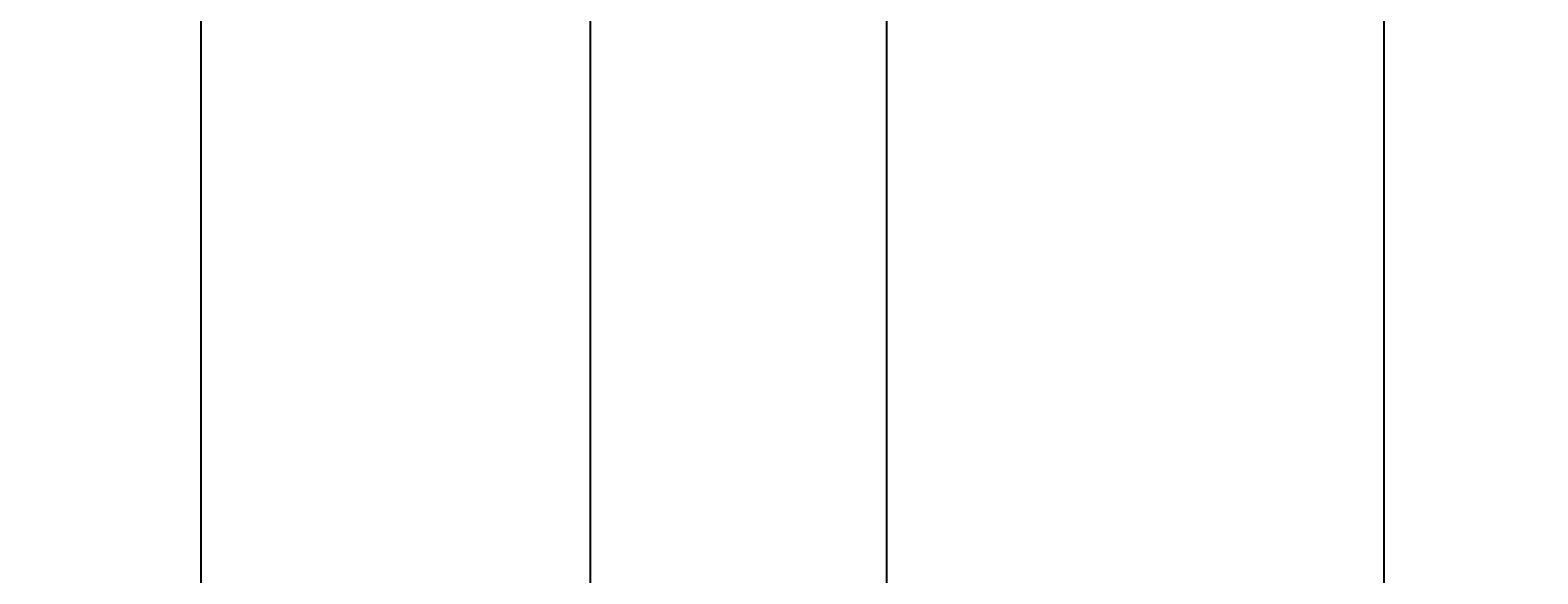
# Model space of a CAD drawing. Units: inches. Extents: x 2231 to 2461, y 2045 to 2455.
# Tile 17 of 95: x 2326 to 2365, y 2099 to 2112. Entities that reach past the tile are written whole.
import ezdxf

# ---------------------------------------------------------------- set-up
doc = ezdxf.new("R2010")
doc.units = ezdxf.units.IN
doc.layers.add('A-ANNO-DIMS', color=2, linetype='Continuous', lineweight=18)
doc.styles.get("Standard").update_dxf_attribs({"font": 'arial.ttf'})
doc.dimstyles.get("Standard").update_dxf_attribs({"dimtxt": 0.18, "dimasz": 0.18, "dimexe": 0.18, "dimexo": 0.0625, "dimgap": 0.09, "dimtad": 0, "dimtih": 1, "dimtoh": 1, "dimdec": 4, "dimzin": 0, "dimdsep": 46, "dimtxsty": 'Standard', "dimcen": 0.09, "dimadec": 0, "dimazin": 0, "dimtfac": 1, "dimtdec": 4, "dimtofl": 0, "dimtmove": 0, "dimatfit": 3, "dimfxl": 1, "dimtolj": 1, "dimtzin": 0, "dimarcsym": 0})

# ---------------------------------------------------------------- blocks, each defined once
blk = doc.blocks.new('*D51')
at = {"layer": 'A-ANNO-DIMS', "color": 0, "lineweight": -2, "transparency": 16777216}
for p, q in [((2258.794, 2306.77), (2258.794, 2044.803)), ((2330.794, 2306.77), (2330.794, 2044.803)), ((2258.974, 2044.983), (2294.576, 2044.983)), ((2330.614, 2044.983), (2295.011, 2044.983))]:
    blk.add_line(p, q, dxfattribs=at)
at = {"layer": 'A-ANNO-DIMS', "color": 0, "transparency": 16777216}
for points in [[(2258.974, 2045.013), (2258.974, 2044.953), (2258.794, 2044.983)], [(2330.614, 2045.013), (2330.614, 2044.953), (2330.794, 2044.983)]]:
    blk.add_solid(points, dxfattribs=at)
at = {"layer": 'Defpoints', "color": 0, "transparency": 16777216}
for p in [(2258.794, 2306.833), (2330.794, 2306.833), (2330.794, 2044.983)]:
    blk.add_point(p, dxfattribs=at)
at = {"layer": 'A-ANNO-DIMS', "color": 0, "transparency": 16777216, "insert": (2294.794, 2044.983), "char_height": 0.18, "attachment_point": 5}
blk.add_mtext('\\A1;72', dxfattribs=at)
blk = doc.blocks.new('*D52')
at = {"layer": 'A-ANNO-DIMS', "color": 0, "lineweight": -2, "transparency": 16777216}
for p, q in [((2330.794, 2306.77), (2330.794, 2044.803)), ((2360.794, 2306.77), (2360.794, 2044.803)), ((2330.974, 2044.983), (2345.575, 2044.983)), ((2360.614, 2044.983), (2346.012, 2044.983))]:
    blk.add_line(p, q, dxfattribs=at)
at = {"layer": 'A-ANNO-DIMS', "color": 0, "transparency": 16777216}
for points in [[(2330.974, 2045.013), (2330.974, 2044.953), (2330.794, 2044.983)], [(2360.614, 2045.013), (2360.614, 2044.953), (2360.794, 2044.983)]]:
    blk.add_solid(points, dxfattribs=at)
at = {"layer": 'Defpoints', "color": 0, "transparency": 16777216}
for p in [(2330.794, 2306.833), (2360.794, 2306.833), (2360.794, 2044.983)]:
    blk.add_point(p, dxfattribs=at)
at = {"layer": 'A-ANNO-DIMS', "color": 0, "transparency": 16777216, "insert": (2345.794, 2044.983), "char_height": 0.18, "attachment_point": 5}
blk.add_mtext('\\A1;30', dxfattribs=at)
blk = doc.blocks.new('*D65')
at = {"layer": 'A-ANNO-DIMS', "color": 0, "lineweight": -2, "transparency": 16777216}
for p, q in [((2285.635, 2189.285), (2285.635, 2044.803)), ((2340.667, 2189.285), (2340.667, 2044.803)), ((2285.815, 2044.983), (2312.758, 2044.983)), ((2340.487, 2044.983), (2313.545, 2044.983))]:
    blk.add_line(p, q, dxfattribs=at)
at = {"layer": 'A-ANNO-DIMS', "color": 0, "transparency": 16777216}
for points in [[(2285.815, 2045.013), (2285.815, 2044.953), (2285.635, 2044.983)], [(2340.487, 2045.013), (2340.487, 2044.953), (2340.667, 2044.983)]]:
    blk.add_solid(points, dxfattribs=at)
at = {"layer": 'Defpoints', "color": 0, "transparency": 16777216}
for p in [(2285.635, 2189.348), (2340.667, 2189.348), (2340.667, 2044.983)]:
    blk.add_point(p, dxfattribs=at)
at = {"layer": 'A-ANNO-DIMS', "color": 0, "transparency": 16777216, "insert": (2313.151, 2044.983), "char_height": 0.18, "attachment_point": 5}
blk.add_mtext('\\A1;55.03', dxfattribs=at)
blk = doc.blocks.new('*D66')
at = {"layer": 'A-ANNO-DIMS', "color": 0, "lineweight": -2, "transparency": 16777216}
for p, q in [((2348.189, 2096.895), (2348.189, 2454.645)), ((2348.369, 2454.465), (2378.167, 2454.465)), ((2408.614, 2454.465), (2378.815, 2454.465)), ((2408.794, 2096.895), (2408.794, 2454.645))]:
    blk.add_line(p, q, dxfattribs=at)
at = {"layer": 'A-ANNO-DIMS', "color": 0, "transparency": 16777216}
for points in [[(2348.369, 2454.495), (2348.369, 2454.435), (2348.189, 2454.465)], [(2408.614, 2454.495), (2408.614, 2454.435), (2408.794, 2454.465)]]:
    blk.add_solid(points, dxfattribs=at)
at = {"layer": 'Defpoints', "color": 0, "transparency": 16777216}
for p in [(2408.794, 2454.465), (2348.189, 2096.833), (2408.794, 2096.833)]:
    blk.add_point(p, dxfattribs=at)
at = {"layer": 'A-ANNO-DIMS', "color": 0, "transparency": 16777216, "insert": (2378.491, 2454.465), "char_height": 0.18, "attachment_point": 5}
blk.add_mtext('\\A1;60.6', dxfattribs=at)
blk = doc.blocks.new('*D69')
at = {"layer": 'A-ANNO-DIMS', "color": 0, "lineweight": -2, "transparency": 16777216}
for p, q in [((2340.667, 2189.285), (2340.667, 2044.803)), ((2394.794, 2186.77), (2394.794, 2044.803)), ((2340.847, 2044.983), (2367.337, 2044.983)), ((2394.614, 2044.983), (2368.124, 2044.983))]:
    blk.add_line(p, q, dxfattribs=at)
at = {"layer": 'A-ANNO-DIMS', "color": 0, "transparency": 16777216}
for points in [[(2340.847, 2045.013), (2340.847, 2044.953), (2340.667, 2044.983)], [(2394.614, 2045.013), (2394.614, 2044.953), (2394.794, 2044.983)]]:
    blk.add_solid(points, dxfattribs=at)
at = {"layer": 'Defpoints', "color": 0, "transparency": 16777216}
for p in [(2340.667, 2189.348), (2394.794, 2186.833), (2394.794, 2044.983)]:
    blk.add_point(p, dxfattribs=at)
at = {"layer": 'A-ANNO-DIMS', "color": 0, "transparency": 16777216, "insert": (2367.73, 2044.983), "char_height": 0.18, "attachment_point": 5}
blk.add_mtext('\\A1;54.13', dxfattribs=at)

msp = doc.modelspace()

# ---------------------------------------------------------------- dimensions: what is measured, and where the dimension line sits
at = {"layer": 'A-ANNO-DIMS'}
for base, p1, p2, override, picture, middle in [((2408.7935, 2454.4653), (2348.1888, 2096.8328), (2408.7935, 2096.8328), {"dimdec": 1, "dimlfac": 1, "dimrnd": 0, "dimzin": 0, "dimdsep": 46, "dimlunit": 2}, '*D66', (2378.4912, 2454.4653)), ((2330.7935, 2044.9825), (2258.7935, 2306.8328), (2330.7935, 2306.8328), {"dimdec": 0, "dimlfac": 1, "dimrnd": 0, "dimzin": 0, "dimdsep": 46, "dimlunit": 2}, '*D51', (2294.7935, 2044.9825)), ((2360.7935, 2044.9825), (2330.7935, 2306.8328), (2360.7935, 2306.8328), {"dimdec": 0, "dimlfac": 1, "dimrnd": 0, "dimzin": 0, "dimdsep": 46, "dimlunit": 2}, '*D52', (2345.7935, 2044.9825)), ((2340.6673, 2044.9825), (2285.6353, 2189.3477), (2340.6673, 2189.3477), {"dimdec": 2, "dimlfac": 1, "dimrnd": 0, "dimzin": 0, "dimdsep": 46, "dimlunit": 2}, '*D65', (2313.1513, 2044.9825)), ((2394.7935, 2044.9825), (2340.6673, 2189.3477), (2394.7935, 2186.8328), {"dimdec": 2, "dimlfac": 1, "dimrnd": 0, "dimzin": 0, "dimdsep": 46, "dimlunit": 2}, '*D69', (2367.7304, 2044.9825))]:
    dim = msp.add_linear_dim(base=base, p1=p1, p2=p2, dimstyle='Standard', override=override, dxfattribs=at)
    dim.commit()
    dim.dimension.update_dxf_attribs({"geometry": picture, "text_midpoint": middle})

doc.saveas('drawing.dxf')
